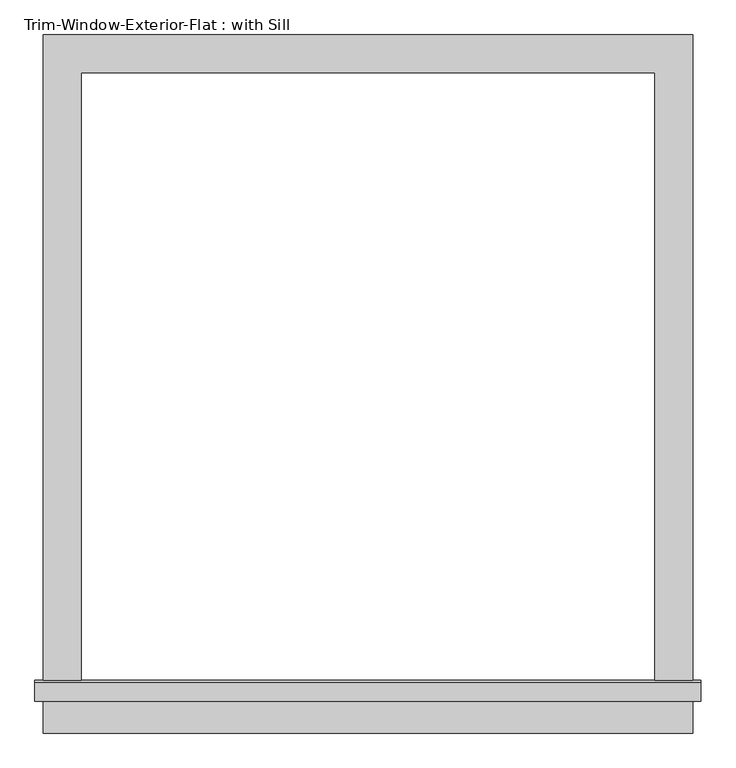
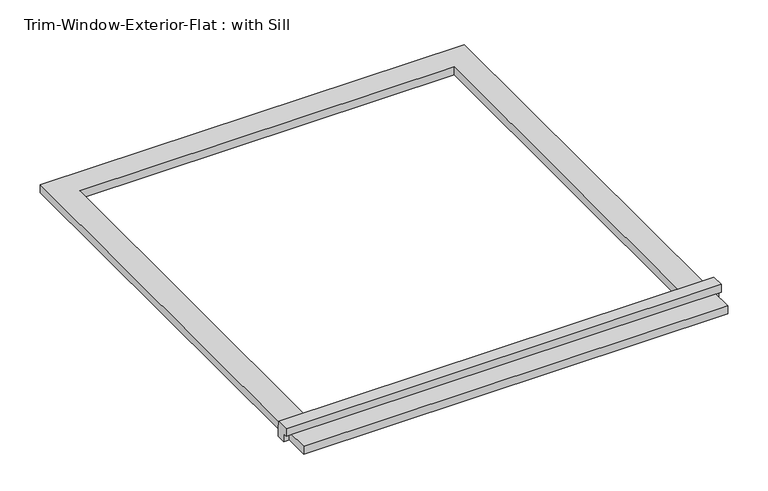
"""IFC4 building model written with IfcOpenShell, lengths in millimetres: proxy geometry, Trim-Window-Exterior-Flat : with Sill."""

from ifc_helpers import new_model, si_unit, frame, origin, origin_with_axes, place, context, project, spatial, polyline, outline, extrude, source, transform, mapped, element, save


def trim_window_exterior_flat_with_sill_41619996(model_context):
    return source(origin(), model_context, "Body", "SweptSolid", [
        extrude(outline(polyline([(488.95, -936.5823709), (488.95, -993.7323709), (-488.95, -993.7323709), (-488.95, -936.5823709), (488.95, -936.5823709)])), origin_with_axes(), (0.0, 0.0, 1.0), 19.05),
        extrude(outline(polyline([(-946.15, 38.1), (-916.8580645, 38.1), (-914.4, 19.05), (-914.4, 0.0), (-936.5823709, 0.0), (-936.5823709, 19.05), (-946.15, 19.05), (-946.15, 38.1)])), frame((-501.65, 0.0, 0.0), z_axis=(1.0, 0.0, 0.0), x_axis=(0.0, 1.0, 0.0)), (0.0, 0.0, 1.0), 1003.3),
        extrude(outline(polyline([(-488.95, 57.15), (488.95, 57.15), (488.95, -914.4), (431.8, -914.4), (431.8, 0.0), (-431.8, 0.0), (-431.8, -914.4), (-488.95, -914.4), (-488.95, 57.15)])), origin_with_axes(), (0.0, 0.0, 1.0), 19.05),
    ])


if __name__ == "__main__":
    model = new_model("IFC4")
    model_context = context("Model", 3, world=origin())
    ifc_project = project(units=[si_unit("LENGTHUNIT", "METRE", prefix="MILLI")], contexts=[model_context])
    site = spatial("IfcSite", under=ifc_project)
    building = spatial("IfcBuilding", under=site)
    placement = place(None, origin())
    trim_window_exterior_flat_with_sill_shape = trim_window_exterior_flat_with_sill_41619996(model_context)
    element("IfcBuildingElementProxy", 1, Name="Trim-Window-Exterior-Flat : with Sill", ObjectType="Trim-Window-Exterior-Flat : with Sill", at=placement, inside=building, context=model_context, shape_type="MappedRepresentation", body=[
        mapped(trim_window_exterior_flat_with_sill_shape, transform((0.0, 0.0, 0.0), x_axis=(1.0, 0.0, 0.0), y_axis=(0.0, 1.0, 0.0), z_axis=(0.0, 0.0, 1.0))),
    ])
    save(model, "model.ifc")

# Revit data of these elements
# Type "Trim-Window-Exterior-Flat : with Sill"
#   Trim Width = 0' - 2 1/4"
#   Trim Thickness_Picture Frame = 0' - 1 1/4"
#   Trim Thickness_with Sill = 0' - 0 3/4"
#   Sill Thickness = 0' - 1 1/4"
#   Opening Width [instance default] = 2' - 0"
#   Opening Height [instance default] = 3' - 0"
#   Default Elevation = 4' - 0"
#   Sill = yes
#   Picture Frame = no
#   Trim Material [instance default] = none
# Element 1 (IfcBuildingElementProxy, "Trim-Window-Exterior-Flat : with Sill")
#   Opening Width = 2' - 10"
#   Trim Material = Clad - White
#   Materials on its faces: "Clad - White"
# Materials
#   "Clad - White": class "Wood", colour RGB 30 30 30, transparency 0, Cost = 0
